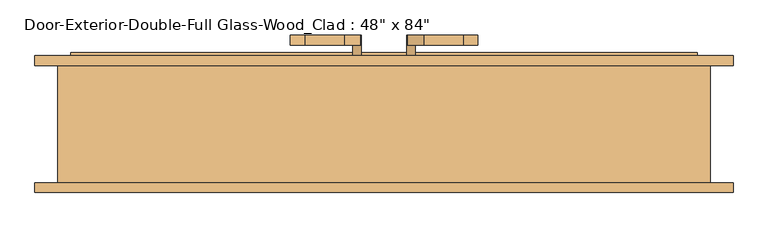
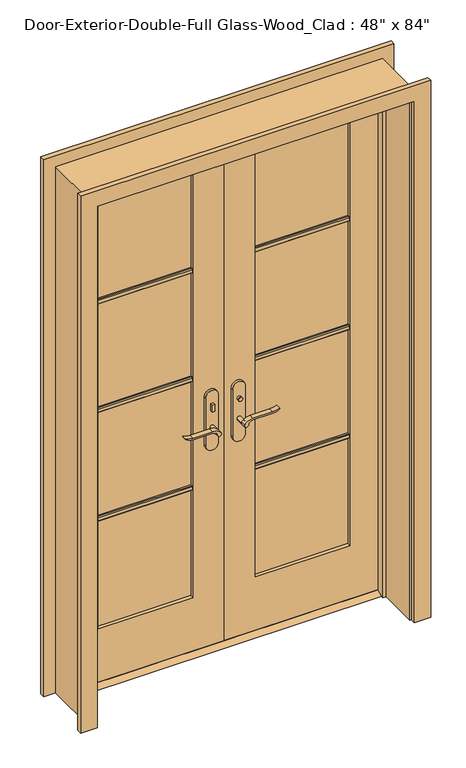
"""IFC4 building model written with IfcOpenShell, lengths in millimetres: door geometry."""

from ifc_helpers import new_model, si_unit, point, frame, frame_2d, origin, place, context, project, spatial, polyline, circle_curve, trimmed, segment, composite_curve, outline, extrude, faceted_brep, source, transform, mapped, element, save


def door_4500b467(model_context):
    return source(origin(), model_context, "Body", "SolidModel", [
        extrude(outline(polyline([(76.2, 12.7), (111.125, 12.7), (136.525, 0.0), (50.8, 0.0), (76.2, 12.7)])), frame((-609.6, 0.0, 0.0), z_axis=(1.0, 0.0, 0.0), x_axis=(0.0, 1.0, 0.0)), (0.0, 0.0, 1.0), 1219.2),
        extrude(outline(polyline([(-47.4019111, 56.2), (-57.4019111, 56.2), (-57.4019111, 66.2), (-47.4019111, 66.2), (-47.4019111, 56.2)])), frame((0.0, 0.0, 981.9), z_axis=(0.0, 0.0, 1.0), x_axis=(1.0, 0.0, 0.0)), (0.0, 0.0, 1.0), 30.0),
        extrude(outline(composite_curve([segment(trimmed(circle_curve(frame_2d((996.9, -52.4019111)), 8.0), [point((996.9, -60.4019111))], [point((996.9, -44.4019111))], False, "CARTESIAN"), True, "CONTINUOUS"), segment(trimmed(circle_curve(frame_2d((996.9, -52.4019111)), 8.0), [point((996.9, -44.4019111))], [point((996.9, -60.4019111))], False, "CARTESIAN"), True, "CONTINUOUS")], self_intersect=False)), frame((0.0, 121.125, 0.0), z_axis=(0.0, 1.0, 0.0), x_axis=(0.0, 0.0, 1.0)), (0.0, 0.0, 1.0), 10.0),
        extrude(outline(composite_curve([segment(trimmed(circle_curve(frame_2d((897.1555521, -76.0694241)), 37.2832219), [point((919.0523287, -45.8937749))], [point((934.4, -77.7693445))], False, "CARTESIAN"), True, "CONTINUOUS"), segment(polyline([(934.4, -77.7693445), (934.4, -154.045502)]), True, "CONTINUOUS"), segment(trimmed(circle_curve(frame_2d((1017.6850638, -153.9791202)), 83.2850902), [point((934.4, -154.045502))], [point((939.4, -182.4019111))], True, "CARTESIAN"), True, "CONTINUOUS"), segment(polyline([(939.4, -182.4019111), (936.6135558, -182.4019111)]), True, "CONTINUOUS"), segment(trimmed(circle_curve(frame_2d((986.6709207, -150.4622499)), 59.3791355), [point((936.6135558, -182.4019111))], [point((927.4, -154.045502))], False, "CARTESIAN"), True, "CONTINUOUS"), segment(polyline([(927.4, -154.045502), (927.4, -77.7881013)]), True, "CONTINUOUS"), segment(trimmed(circle_curve(frame_2d((909.2738613, -77.7881013)), 18.1261387), [point((927.4, -77.7881013))], [point((914.4, -60.4019111))], True, "CARTESIAN"), True, "CONTINUOUS"), segment(trimmed(circle_curve(frame_2d((914.4, -52.4019111)), 8.0), [point((914.4, -60.4019111))], [point((919.0523287, -45.8937749))], False, "CARTESIAN"), True, "CONTINUOUS")], self_intersect=False)), frame((0.0, 16.2, 0.0), z_axis=(0.0, 1.0, 0.0), x_axis=(0.0, 0.0, 1.0)), (0.0, 0.0, 1.0), 20.0),
        extrude(outline(composite_curve([segment(trimmed(circle_curve(frame_2d((914.4, -52.4019111)), 8.0), [point((914.3999903, -60.4019111))], [point((919.0523287, -45.8937749))], False, "CARTESIAN"), True, "CONTINUOUS"), segment(trimmed(circle_curve(frame_2d((897.1555521, -76.0694241)), 37.2832219), [point((919.0523287, -45.8937749))], [point((934.4, -77.7693445))], False, "CARTESIAN"), True, "CONTINUOUS"), segment(polyline([(934.4, -77.7693445), (934.4, -154.045502)]), True, "CONTINUOUS"), segment(trimmed(circle_curve(frame_2d((1017.6850638, -153.9791202)), 83.2850902), [point((934.4, -154.045502))], [point((939.4, -182.4019111))], True, "CARTESIAN"), True, "CONTINUOUS"), segment(polyline([(939.4, -182.4019111), (936.6135558, -182.4019111)]), True, "CONTINUOUS"), segment(trimmed(circle_curve(frame_2d((986.6709207, -150.4622499)), 59.3791355), [point((936.6135558, -182.4019111))], [point((927.4, -154.045502))], False, "CARTESIAN"), True, "CONTINUOUS"), segment(polyline([(927.4, -154.045502), (927.4, -77.788099)]), True, "CONTINUOUS"), segment(trimmed(circle_curve(frame_2d((909.2738682, -77.788099)), 18.1261318), [point((927.4, -77.788099))], [point((914.3999903, -60.4019111))], True, "CARTESIAN"), True, "CONTINUOUS")], self_intersect=False)), frame((0.0, 151.125, 0.0), z_axis=(0.0, 1.0, 0.0), x_axis=(0.0, 0.0, 1.0)), (0.0, 0.0, 1.0), 20.0),
        extrude(outline(composite_curve([segment(trimmed(circle_curve(frame_2d((914.4, -52.4019111)), 8.0), [point((914.4, -60.4019111))], [point((914.4, -44.4019111))], False, "CARTESIAN"), True, "CONTINUOUS"), segment(trimmed(circle_curve(frame_2d((914.4, -52.4019111)), 8.0), [point((914.4, -44.4019111))], [point((914.4, -60.4019111))], False, "CARTESIAN"), True, "CONTINUOUS")], self_intersect=False)), frame((0.0, 36.2, 0.0), z_axis=(0.0, 1.0, 0.0), x_axis=(0.0, 0.0, 1.0)), (0.0, 0.0, 1.0), 30.0),
        extrude(outline(composite_curve([segment(trimmed(circle_curve(frame_2d((914.4, -52.4019111)), 8.0), [point((914.4, -60.4019111))], [point((914.4, -44.4019111))], False, "CARTESIAN"), True, "CONTINUOUS"), segment(trimmed(circle_curve(frame_2d((914.4, -52.4019111)), 8.0), [point((914.4, -44.4019111))], [point((914.4, -60.4019111))], False, "CARTESIAN"), True, "CONTINUOUS")], self_intersect=False)), frame((0.0, 121.125, 0.0), z_axis=(0.0, 1.0, 0.0), x_axis=(0.0, 0.0, 1.0)), (0.0, 0.0, 1.0), 30.0),
        extrude(outline(composite_curve([segment(polyline([(844.4, -27.4019111), (1039.4, -27.4019111)]), True, "CONTINUOUS"), segment(trimmed(circle_curve(frame_2d((1039.4, -52.4019111)), 25.0), [point((1039.4, -27.4019111))], [point((1039.4, -77.4019111))], False, "CARTESIAN"), True, "CONTINUOUS"), segment(polyline([(1039.4, -77.4019111), (844.4, -77.4019111)]), True, "CONTINUOUS"), segment(trimmed(circle_curve(frame_2d((844.4, -52.4019111)), 25.0), [point((844.4, -77.4019111))], [point((844.4, -27.4019111))], False, "CARTESIAN"), True, "CONTINUOUS")], self_intersect=False)), frame((0.0, 66.2, 0.0), z_axis=(0.0, 1.0, 0.0), x_axis=(0.0, 0.0, 1.0)), (0.0, 0.0, 1.0), 10.0),
        extrude(outline(composite_curve([segment(polyline([(844.4, -27.4019111), (1039.4, -27.4019111)]), True, "CONTINUOUS"), segment(trimmed(circle_curve(frame_2d((1039.4, -52.4019111)), 25.0), [point((1039.4, -27.4019111))], [point((1039.4, -77.4019111))], False, "CARTESIAN"), True, "CONTINUOUS"), segment(polyline([(1039.4, -77.4019111), (844.4, -77.4019111)]), True, "CONTINUOUS"), segment(trimmed(circle_curve(frame_2d((844.4, -52.4019111)), 25.0), [point((844.4, -77.4019111))], [point((844.4, -27.4019111))], False, "CARTESIAN"), True, "CONTINUOUS")], self_intersect=False)), frame((0.0, 111.125, 0.0), z_axis=(0.0, 1.0, 0.0), x_axis=(0.0, 0.0, 1.0)), (0.0, 0.0, 1.0), 10.0),
        extrude(outline(polyline([(47.3875, 131.125), (57.3875, 131.125), (57.3875, 121.125), (47.3875, 121.125), (47.3875, 131.125)])), frame((0.0, 0.0, 981.9), z_axis=(0.0, 0.0, 1.0), x_axis=(1.0, 0.0, 0.0)), (0.0, 0.0, 1.0), 30.0),
        extrude(outline(composite_curve([segment(trimmed(circle_curve(frame_2d((996.9, 52.3875)), 8.0), [point((996.9, 60.3875))], [point((996.9, 44.3875))], False, "CARTESIAN"), True, "CONTINUOUS"), segment(trimmed(circle_curve(frame_2d((996.9, 52.3875)), 8.0), [point((996.9, 44.3875))], [point((996.9, 60.3875))], False, "CARTESIAN"), True, "CONTINUOUS")], self_intersect=False)), frame((0.0, 56.2, 0.0), z_axis=(0.0, 1.0, 0.0), x_axis=(0.0, 0.0, 1.0)), (0.0, 0.0, 1.0), 10.0),
        extrude(outline(composite_curve([segment(trimmed(circle_curve(frame_2d((914.4, 52.3875)), 8.0), [point((919.0523287, 45.8793637))], [point((914.4, 60.3875))], False, "CARTESIAN"), True, "CONTINUOUS"), segment(trimmed(circle_curve(frame_2d((909.2738613, 77.7736901)), 18.1261387), [point((914.4, 60.3875))], [point((927.4, 77.7736901))], True, "CARTESIAN"), True, "CONTINUOUS"), segment(polyline([(927.4, 77.7736901), (927.4, 154.0310909)]), True, "CONTINUOUS"), segment(trimmed(circle_curve(frame_2d((986.6709207, 150.4478388)), 59.3791355), [point((927.4, 154.0310909))], [point((936.6135558, 182.3875))], False, "CARTESIAN"), True, "CONTINUOUS"), segment(polyline([(936.6135558, 182.3875), (939.4, 182.3875)]), True, "CONTINUOUS"), segment(trimmed(circle_curve(frame_2d((1017.6850638, 153.9647091)), 83.2850902), [point((939.4, 182.3875))], [point((934.4, 154.0310909))], True, "CARTESIAN"), True, "CONTINUOUS"), segment(polyline([(934.4, 154.0310909), (934.4, 77.7549333)]), True, "CONTINUOUS"), segment(trimmed(circle_curve(frame_2d((897.1555521, 76.0550129)), 37.2832219), [point((934.4, 77.7549333))], [point((919.0523287, 45.8793637))], False, "CARTESIAN"), True, "CONTINUOUS")], self_intersect=False)), frame((0.0, 151.125, 0.0), z_axis=(0.0, 1.0, 0.0), x_axis=(0.0, 0.0, 1.0)), (0.0, 0.0, 1.0), 20.0),
        extrude(outline(composite_curve([segment(trimmed(circle_curve(frame_2d((909.2738682, 77.7736878)), 18.1261318), [point((914.3999903, 60.3875))], [point((927.4, 77.7736878))], True, "CARTESIAN"), True, "CONTINUOUS"), segment(polyline([(927.4, 77.7736878), (927.4, 154.0310909)]), True, "CONTINUOUS"), segment(trimmed(circle_curve(frame_2d((986.6709207, 150.4478388)), 59.3791355), [point((927.4, 154.0310909))], [point((936.6135558, 182.3875))], False, "CARTESIAN"), True, "CONTINUOUS"), segment(polyline([(936.6135558, 182.3875), (939.4, 182.3875)]), True, "CONTINUOUS"), segment(trimmed(circle_curve(frame_2d((1017.6850638, 153.9647091)), 83.2850902), [point((939.4, 182.3875))], [point((934.4, 154.0310909))], True, "CARTESIAN"), True, "CONTINUOUS"), segment(polyline([(934.4, 154.0310909), (934.4, 77.7549333)]), True, "CONTINUOUS"), segment(trimmed(circle_curve(frame_2d((897.1555521, 76.0550129)), 37.2832219), [point((934.4, 77.7549333))], [point((919.0523287, 45.8793637))], False, "CARTESIAN"), True, "CONTINUOUS"), segment(trimmed(circle_curve(frame_2d((914.4, 52.3875)), 8.0), [point((919.0523287, 45.8793637))], [point((914.3999903, 60.3875))], False, "CARTESIAN"), True, "CONTINUOUS")], self_intersect=False)), frame((0.0, 16.2, 0.0), z_axis=(0.0, 1.0, 0.0), x_axis=(0.0, 0.0, 1.0)), (0.0, 0.0, 1.0), 20.0),
        extrude(outline(composite_curve([segment(trimmed(circle_curve(frame_2d((914.4, 52.3875)), 8.0), [point((914.4, 60.3875))], [point((914.4, 44.3875))], False, "CARTESIAN"), True, "CONTINUOUS"), segment(trimmed(circle_curve(frame_2d((914.4, 52.3875)), 8.0), [point((914.4, 44.3875))], [point((914.4, 60.3875))], False, "CARTESIAN"), True, "CONTINUOUS")], self_intersect=False)), frame((0.0, 121.125, 0.0), z_axis=(0.0, 1.0, 0.0), x_axis=(0.0, 0.0, 1.0)), (0.0, 0.0, 1.0), 30.0),
        extrude(outline(composite_curve([segment(trimmed(circle_curve(frame_2d((914.4, 52.3875)), 8.0), [point((914.4, 60.3875))], [point((914.4, 44.3875))], False, "CARTESIAN"), True, "CONTINUOUS"), segment(trimmed(circle_curve(frame_2d((914.4, 52.3875)), 8.0), [point((914.4, 44.3875))], [point((914.4, 60.3875))], False, "CARTESIAN"), True, "CONTINUOUS")], self_intersect=False)), frame((0.0, 36.2, 0.0), z_axis=(0.0, 1.0, 0.0), x_axis=(0.0, 0.0, 1.0)), (0.0, 0.0, 1.0), 30.0),
        extrude(outline(composite_curve([segment(trimmed(circle_curve(frame_2d((844.4, 52.3875)), 25.0), [point((844.4, 27.3875))], [point((844.4, 77.3875))], False, "CARTESIAN"), True, "CONTINUOUS"), segment(polyline([(844.4, 77.3875), (1039.4, 77.3875)]), True, "CONTINUOUS"), segment(trimmed(circle_curve(frame_2d((1039.4, 52.3875)), 25.0), [point((1039.4, 77.3875))], [point((1039.4, 27.3875))], False, "CARTESIAN"), True, "CONTINUOUS"), segment(polyline([(1039.4, 27.3875), (844.4, 27.3875)]), True, "CONTINUOUS")], self_intersect=False)), frame((0.0, 111.125, 0.0), z_axis=(0.0, 1.0, 0.0), x_axis=(0.0, 0.0, 1.0)), (0.0, 0.0, 1.0), 10.0),
        extrude(outline(composite_curve([segment(trimmed(circle_curve(frame_2d((844.4, 52.3875)), 25.0), [point((844.4, 27.3875))], [point((844.4, 77.3875))], False, "CARTESIAN"), True, "CONTINUOUS"), segment(polyline([(844.4, 77.3875), (1039.4, 77.3875)]), True, "CONTINUOUS"), segment(trimmed(circle_curve(frame_2d((1039.4, 52.3875)), 25.0), [point((1039.4, 77.3875))], [point((1039.4, 27.3875))], False, "CARTESIAN"), True, "CONTINUOUS"), segment(polyline([(1039.4, 27.3875), (844.4, 27.3875)]), True, "CONTINUOUS")], self_intersect=False)), frame((0.0, 66.2, 0.0), z_axis=(0.0, 1.0, 0.0), x_axis=(0.0, 0.0, 1.0)), (0.0, 0.0, 1.0), 10.0),
        extrude(outline(polyline([(90.17, 1578.371875), (90.17, 1559.321875), (83.82, 1559.321875), (80.645, 1562.496875), (80.645, 1575.196875), (83.82, 1578.371875), (90.17, 1578.371875)])), frame((120.65, 0.0, 0.0), z_axis=(1.0, 0.0, 0.0), x_axis=(0.0, 1.0, 0.0)), (0.0, 0.0, 1.0), 368.3),
        extrude(outline(polyline([(90.17, 1132.68125), (90.17, 1113.63125), (83.82, 1113.63125), (80.645, 1116.80625), (80.645, 1129.50625), (83.82, 1132.68125), (90.17, 1132.68125)])), frame((120.65, 0.0, 0.0), z_axis=(1.0, 0.0, 0.0), x_axis=(0.0, 1.0, 0.0)), (0.0, 0.0, 1.0), 368.3),
        extrude(outline(polyline([(90.17, 686.990625), (90.17, 667.940625), (83.82, 667.940625), (80.645, 671.115625), (80.645, 683.815625), (83.82, 686.990625), (90.17, 686.990625)])), frame((120.65, 0.0, 0.0), z_axis=(1.0, 0.0, 0.0), x_axis=(0.0, 1.0, 0.0)), (0.0, 0.0, 1.0), 368.3),
        extrude(outline(polyline([(97.155, 1578.371875), (103.505, 1578.371875), (106.68, 1575.196875), (106.68, 1562.496875), (103.505, 1559.321875), (97.155, 1559.321875), (97.155, 1578.371875)])), frame((-488.95, 0.0, 0.0), z_axis=(1.0, 0.0, 0.0), x_axis=(0.0, 1.0, 0.0)), (0.0, 0.0, 1.0), 368.3),
        extrude(outline(polyline([(97.155, 1132.68125), (103.505, 1132.68125), (106.68, 1129.50625), (106.68, 1116.80625), (103.505, 1113.63125), (97.155, 1113.63125), (97.155, 1132.68125)])), frame((-488.95, 0.0, 0.0), z_axis=(1.0, 0.0, 0.0), x_axis=(0.0, 1.0, 0.0)), (0.0, 0.0, 1.0), 368.3),
        extrude(outline(polyline([(97.155, 686.990625), (103.505, 686.990625), (106.68, 683.815625), (106.68, 671.115625), (103.505, 667.940625), (97.155, 667.940625), (97.155, 686.990625)])), frame((-488.95, 0.0, 0.0), z_axis=(1.0, 0.0, 0.0), x_axis=(0.0, 1.0, 0.0)), (0.0, 0.0, 1.0), 368.3),
        extrude(outline(polyline([(97.155, 1578.371875), (103.505, 1578.371875), (106.68, 1575.196875), (106.68, 1562.496875), (103.505, 1559.321875), (97.155, 1559.321875), (97.155, 1578.371875)])), frame((120.65, 0.0, 0.0), z_axis=(1.0, 0.0, 0.0), x_axis=(0.0, 1.0, 0.0)), (0.0, 0.0, 1.0), 368.3),
        extrude(outline(polyline([(97.155, 1132.68125), (103.505, 1132.68125), (106.68, 1129.50625), (106.68, 1116.80625), (103.505, 1113.63125), (97.155, 1113.63125), (97.155, 1132.68125)])), frame((120.65, 0.0, 0.0), z_axis=(1.0, 0.0, 0.0), x_axis=(0.0, 1.0, 0.0)), (0.0, 0.0, 1.0), 368.3),
        extrude(outline(polyline([(97.155, 686.990625), (103.505, 686.990625), (106.68, 683.815625), (106.68, 671.115625), (103.505, 667.940625), (97.155, 667.940625), (97.155, 686.990625)])), frame((120.65, 0.0, 0.0), z_axis=(1.0, 0.0, 0.0), x_axis=(0.0, 1.0, 0.0)), (0.0, 0.0, 1.0), 368.3),
        extrude(outline(polyline([(90.17, 1578.371875), (90.17, 1559.321875), (83.82, 1559.321875), (80.645, 1562.496875), (80.645, 1575.196875), (83.82, 1578.371875), (90.17, 1578.371875)])), frame((-488.95, 0.0, 0.0), z_axis=(1.0, 0.0, 0.0), x_axis=(0.0, 1.0, 0.0)), (0.0, 0.0, 1.0), 368.3),
        extrude(outline(polyline([(90.17, 1132.68125), (90.17, 1113.63125), (83.82, 1113.63125), (80.645, 1116.80625), (80.645, 1129.50625), (83.82, 1132.68125), (90.17, 1132.68125)])), frame((-488.95, 0.0, 0.0), z_axis=(1.0, 0.0, 0.0), x_axis=(0.0, 1.0, 0.0)), (0.0, 0.0, 1.0), 368.3),
        extrude(outline(polyline([(90.17, 686.990625), (90.17, 667.940625), (83.82, 667.940625), (80.645, 671.115625), (80.645, 683.815625), (83.82, 686.990625), (90.17, 686.990625)])), frame((-488.95, 0.0, 0.0), z_axis=(1.0, 0.0, 0.0), x_axis=(0.0, 1.0, 0.0)), (0.0, 0.0, 1.0), 368.3),
        extrude(outline(polyline([(0.0, 615.95), (0.0, 679.45), (2203.45, 679.45), (2203.45, -679.45), (0.0, -679.45), (0.0, -615.95), (2139.95, -615.95), (2139.95, 615.95), (0.0, 615.95)])), frame((0.0, 111.125, 0.0), z_axis=(0.0, 1.0, 0.0), x_axis=(0.0, 0.0, 1.0)), (0.0, 0.0, 1.0), 19.05),
        extrude(outline(polyline([(0.0, 615.95), (0.0, 679.45), (2203.45, 679.45), (2203.45, -679.45), (0.0, -679.45), (0.0, -615.95), (2139.95, -615.95), (2139.95, 615.95), (0.0, 615.95)])), frame((0.0, -136.525, 0.0), z_axis=(0.0, 1.0, 0.0), x_axis=(0.0, 0.0, 1.0)), (0.0, 0.0, 1.0), 19.05),
        extrude(outline(polyline([(12.7, 609.6), (2133.6, 609.6), (2133.6, 1.5875), (12.7, 1.5875), (12.7, 609.6)]), holes=[polyline([(2014.5375, 120.65), (2014.5375, 488.95), (231.775, 488.95), (231.775, 120.65), (2014.5375, 120.65)])]), frame((0.0, 76.2, 0.0), z_axis=(0.0, 1.0, 0.0), x_axis=(0.0, 0.0, 1.0)), (0.0, 0.0, 1.0), 34.925),
        extrude(outline(polyline([(2133.6, -609.6), (12.7, -609.6), (12.7, -1.6019111), (2133.6, -1.6019111), (2133.6, -609.6)]), holes=[polyline([(231.775, -488.95), (2014.5375, -488.95), (2014.5375, -120.65), (231.775, -120.65), (231.775, -488.95)])]), frame((0.0, 76.2, 0.0), z_axis=(0.0, 1.0, 0.0), x_axis=(0.0, 0.0, 1.0)), (0.0, 0.0, 1.0), 34.925),
        faceted_brep([(635.0, 111.125, 0.0), (635.0, -117.475, 0.0), (609.6, -117.475, 0.0), (609.6, 41.275, 0.0), (596.9, 41.275, 0.0), (596.9, 76.2, 0.0), (609.6, 76.2, 0.0), (609.6, 111.125, 0.0), (635.0, 111.125, 2159.0), (635.0, -117.475, 2159.0), (-635.0, -117.475, 2159.0), (-635.0, -117.475, 0.0), (-609.6, -117.475, 0.0), (-609.6, -117.475, 2133.6), (609.6, -117.475, 2133.6), (609.6, 41.275, 2133.6), (-609.6, 41.275, 2133.6), (-609.6, 41.275, 0.0), (-596.9, 41.275, 0.0), (-596.9, 41.275, 2120.9), (596.9, 41.275, 2120.9), (596.9, 76.2, 2120.9), (1.5875, 76.2, 2120.9), (-1.6019111, 76.2, 2120.9), (-596.9, 76.2, 2120.9), (-596.9, 76.2, 0.0), (-609.6, 76.2, 0.0), (-609.6, 76.2, 2133.6), (-1.6019111, 76.2, 2133.6), (1.5875, 76.2, 2133.6), (609.6, 76.2, 2133.6), (609.6, 111.125, 2133.6), (1.5875, 111.125, 2133.6), (-1.6019111, 111.125, 2133.6), (-609.6, 111.125, 2133.6), (-609.6, 111.125, 0.0), (-635.0, 111.125, 0.0), (-635.0, 111.125, 2159.0)], [[[0, 1, 2, 3, 4, 5, 6, 7]], [[1, 0, 8, 9]], [[2, 1, 9, 10, 11, 12, 13, 14]], [[3, 2, 14, 15]], [[4, 3, 15, 16, 17, 18, 19, 20]], [[5, 4, 20, 21]], [[6, 5, 21, 22, 23, 24, 25, 26, 27, 28, 29, 30]], [[7, 6, 30, 31]], [[0, 7, 31, 32, 33, 34, 35, 36, 37, 8]], [[9, 8, 37, 10]], [[14, 13, 16, 15]], [[20, 19, 24, 23, 22, 21]], [[31, 30, 29, 28, 27, 34, 33, 32]], [[12, 11, 36, 35, 26, 25, 18, 17]], [[11, 10, 37, 36]], [[13, 12, 17, 16]], [[19, 18, 25, 24]], [[27, 26, 35, 34]]]),
        extrude(outline(polyline([(488.95, 90.17), (120.65, 90.17), (120.65, 97.155), (488.95, 97.155), (488.95, 90.17)])), frame((0.0, 0.0, 231.775), z_axis=(0.0, 0.0, 1.0), x_axis=(1.0, 0.0, 0.0)), (0.0, 0.0, 1.0), 1782.7625),
        extrude(outline(polyline([(-120.65, 90.17), (-488.95, 90.17), (-488.95, 97.155), (-120.65, 97.155), (-120.65, 90.17)])), frame((0.0, 0.0, 231.775), z_axis=(0.0, 0.0, 1.0), x_axis=(1.0, 0.0, 0.0)), (0.0, 0.0, 1.0), 1782.7625),
    ])


if __name__ == "__main__":
    model = new_model("IFC4")
    model_context = context("Model", 3, world=origin())
    ifc_project = project(units=[si_unit("LENGTHUNIT", "METRE", prefix="MILLI")], contexts=[model_context])
    site = spatial("IfcSite", under=ifc_project)
    building = spatial("IfcBuilding", under=site)
    placement = place(None, origin())
    door_shape = door_4500b467(model_context)
    element("IfcDoor", 1, ObjectType="Door-Exterior-Double-Full Glass-Wood_Clad : 48\" x 84\"", at=placement, inside=building, context=model_context, shape_type="MappedRepresentation", body=[
        mapped(door_shape, transform((0.0, 0.0, 0.0), x_axis=(1.0, 0.0, 0.0), y_axis=(0.0, 1.0, 0.0), z_axis=(0.0, 0.0, 1.0))),
    ])
    save(model, "model.ifc")

# Revit data of these elements
# Type "Door-Exterior-Double-Full Glass-Wood_Clad : 48\" x 84\""
#   Type Mark = "9"
#   Assembly Code = "B2030100"
#   Analytic Construction = "French door, wood frame with double glass"
#   Top Rail = 0' - 4 11/16"
#   Threshold Offset [instance default] = 0' - 0 1/2"
#   Thickness = 0' - 1 3/8"
#   Thermal Resistance (R) = 1.9158 (h·ft²·°F)/BTU
#   Swing Angle [instance default] = 90.00°
#   Stiles = 0' - 4 3/4"
#   Rough Width = 4' - 2"
#   Rough Height = 7' - 1"
#   Panel Width = 2' - 0"
#   Door Offset [instance default] = 0' - 0"
#   Height = 7' - 0"
#   Width = 4' - 0"
#   Heat Transfer Coefficient (U) = 0.5220 BTU/(h·ft²·°F)
#   Bottom Rail = 0' - 9 1/8"
#   Exterior Trim [instance default] = yes
#   Threshold [instance default] = yes
#   Show Grill [instance default] = yes
#   Function = 1
#   Trim Material = Cherry
#   Threshold Material = Cherry
#   Panel Material = Cherry
#   Glazing = Glass
#   Frame Material = Cherry
#   Door Handle Material = Aluminum
#   Visual Light Transmittance = 0
#   Solar Heat Gain Coefficient = 0
#   Wall Closure = (empty or 0)
#   Construction Type = (empty or 0)
# Element 1 (IfcDoor, "Door-Exterior-Double-Full Glass-Wood_Clad : 48\" x 84\"")
#   Materials on its faces: "Cherry", "Aluminum", "Glass"
# Materials
#   "Cherry": class "Wood", colour RGB 226 177 128, transparency 0, Description = "Prunus Serotina", Cost = 0
#   "Glass": class "Glass", colour RGB 0 128 192, transparency 0.75, Description = "Soda Lime Glass", Cost = 0
#   "Aluminum": class "Metal", colour RGB 247 247 247, transparency 0, Description = "Aluminum 6061", Cost = 0
